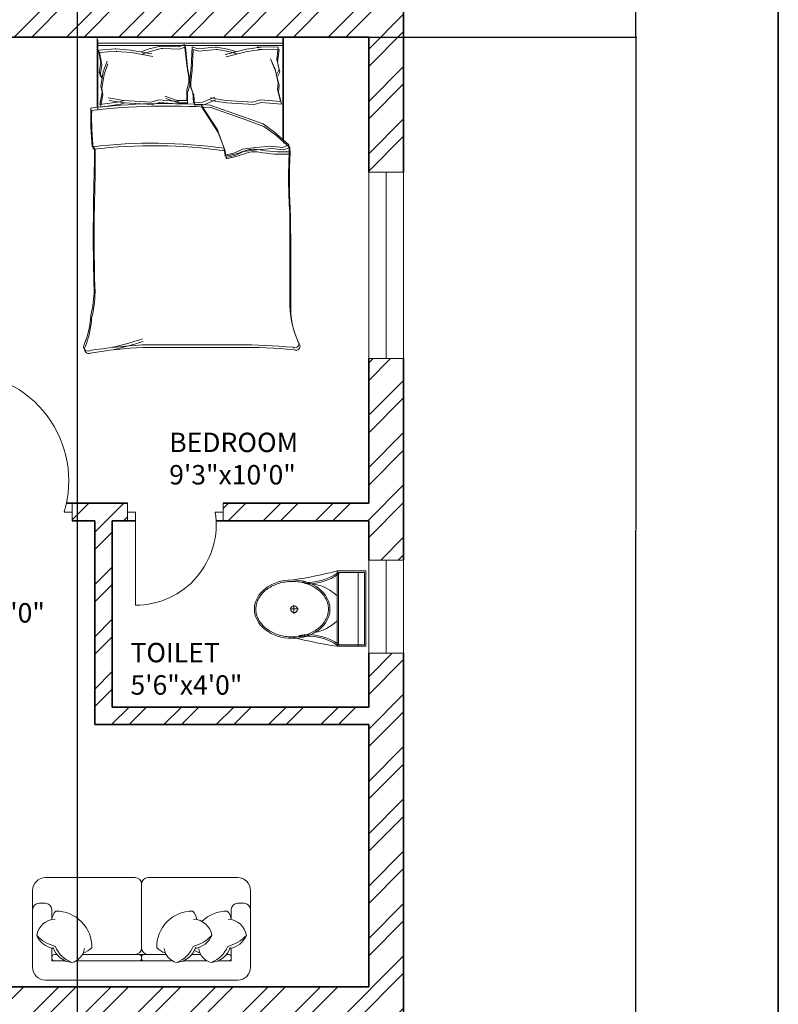
# Model space of a CAD drawing. Units: inches. Extents: x 2552 to 3217, y 1417 to 2737.
# Tile 15 of 25: x 3022 to 3217, y 2138 to 2392. Entities that reach past the tile are written whole.
import ezdxf

# ---------------------------------------------------------------- set-up
doc = ezdxf.new("R2010")
doc.units = ezdxf.units.IN
for name, color, linetype, lineweight in [('A-ANNO-DIMS', 2, 'Continuous', 18), ('A-ANNO-TTLB', 7, 'Continuous', 35), ('A-AREA-IDEN', 7, 'Continuous', 18), ('A-DOOR', 21, 'Continuous', 18), ('A-FLOR-FIXT', 8, 'Continuous', 18), ('A-FURN', 8, 'Continuous', 13), ('A-GLAZ', 161, 'Continuous', 18), ('A-WALL', 7, 'Continuous', 35), ('A-WALL-PATT', 217, 'Continuous', 13)]:
    doc.layers.add(name, color=color, linetype=linetype, lineweight=lineweight)
doc.styles.get("Standard").update_dxf_attribs({"font": 'arial.ttf'})
doc.dimstyles.get("Standard").update_dxf_attribs({"dimtxt": 0.18, "dimasz": 0.18, "dimexe": 0.18, "dimexo": 0.0625, "dimgap": 0.09, "dimtad": 0, "dimtih": 1, "dimtoh": 1, "dimdec": 4, "dimzin": 0, "dimdsep": 46, "dimtxsty": 'Standard', "dimcen": 0.09, "dimadec": 0, "dimazin": 0, "dimtfac": 1, "dimtdec": 4, "dimtofl": 0, "dimtmove": 0, "dimatfit": 3, "dimfxl": 1, "dimtolj": 1, "dimtzin": 0, "dimarcsym": 0})

# ---------------------------------------------------------------- blocks, each defined once
blk = doc.blocks.new('A$C31115884')
for p, q in [((283.1, 497.7), (223.4, 497.7)), ((257.5, 466.4), (257.5, 523.2)), ((0, 200), (0, 0)), ((520, 200), (0, 200)), ((10, 190), (10, 10)), ((510, 190), (10, 190)), ((510, 10), (510, 190)), ((520, 0), (520, 200)), ((510, 54.5), (0, 54.5)), ((10, 10), (510, 10)), ((0, 0), (520, 0))]:
    blk.add_line(p, q)
blk.add_circle((255.6, 496.4), 23.6)
for centre, radius, start, end in [((2777.7, -204.6), 2807, 165.4549, 171.71327), ((3237, 905), 2807, 188.28673, 194.5451), ((-294.5, 403.3), 364.7, 324.20913, 9.34987), ((-294.5, 403.3), 374.7, 324.20913, 9.34987), ((139.5, 406.2), 293.5, 315.84364, 2.65635), ((805.8, 403.3), 374.7, 179.20365, 215.79087), ((805.8, 403.3), 364.7, 170.65013, 215.79087), ((383.6, 406.2), 293.5, 190.27735, 224.15636)]:
    blk.add_arc(centre, radius, start, end)
blk.add_ellipse((256.2, 509.9), major_axis=(0, -260.7), ratio=0.772727)
blk.add_open_spline([(256.2, 259.2), (263.1, 259.2), (270, 259.7), (287.8, 262.3), (298.7, 265.1), (319.9, 273.1), (330.2, 278.4), (350.1, 291.1), (359.7, 298.7), (377.7, 315.9), (386.2, 325.5), (401.7, 346.6), (408.8, 358.1), (421.3, 382.5), (426.8, 395.5), (435.9, 422.4), (439.5, 436.4), (444.8, 465.1), (446.5, 479.7), (447.9, 509.2), (447.6, 524), (445, 553.3), (442.7, 567.8), (436.3, 596), (432.1, 609.7), (421.9, 636), (416, 648.6), (402.5, 672.1), (395, 683), (378.6, 703), (369.8, 712.1), (351.1, 728), (341.3, 734.8), (320.9, 746.2), (310.4, 750.7), (288.9, 757.3), (278, 759.4), (256, 761), (245, 760.6), (223.1, 757.2), (212.3, 754.3), (191.1, 746.1), (180.8, 740.7), (160.9, 727.8), (151.4, 720.1), (133.5, 702.7), (125.1, 693), (109.6, 671.7), (102.6, 660.2), (90.2, 635.7), (84.9, 622.7), (76, 595.6), (72.4, 581.6), (67.2, 552.9), (65.6, 538.2), (64.4, 508.8), (64.8, 494), (67.5, 464.7), (69.9, 450.2), (76.6, 422), (80.8, 408.3), (91.1, 382.2), (97.2, 369.7), (110.8, 346.3), (118.4, 335.4), (134.8, 315.6), (143.7, 306.7), (162.4, 290.9), (172.3, 284.2), (192.8, 273), (203.3, 268.6), (224.8, 262.2), (235.8, 260.2), (249.9, 259.3), (253, 259.2), (256.2, 259.2)], degree=3, knots=[0, 0, 0, 0, 0.110105, 0.110105, 0.285049, 0.285049, 0.459994, 0.459994, 0.634938, 0.634938, 0.809882, 0.809882, 0.984827, 0.984827, 1.159771, 1.159771, 1.334715, 1.334715, 1.50966, 1.50966, 1.684604, 1.684604, 1.859549, 1.859549, 2.034493, 2.034493, 2.209437, 2.209437, 2.384382, 2.384382, 2.559326, 2.559326, 2.73427, 2.73427, 2.909215, 2.909215, 3.084159, 3.084159, 3.259103, 3.259103, 3.434048, 3.434048, 3.608992, 3.608992, 3.783936, 3.783936, 3.958881, 3.958881, 4.133825, 4.133825, 4.30877, 4.30877, 4.483714, 4.483714, 4.658658, 4.658658, 4.833603, 4.833603, 5.008547, 5.008547, 5.183491, 5.183491, 5.358436, 5.358436, 5.53338, 5.53338, 5.708324, 5.708324, 5.883269, 5.883269, 6.058213, 6.058213, 6.233158, 6.233158, 6.283185, 6.283185, 6.283185, 6.283185])
blk = doc.blocks.new('BED-DOUBLE')
for p, q in [((3.47, 63.33), (3.47, 81.44)), ((3.47, 81.44), (51.49, 81.44)), ((3.48, 63.33), (3.48, 81.44)), ((51.27, 81.44), (51.27, 54.83)), ((51.27, 81.44), (51.27, 54.83)), ((51.49, 81.44), (51.49, 80.8)), ((3.47, 79.91), (51.27, 79.91)), ((3.48, 79.91), (51.27, 79.91)), ((3.7, 62.69), (3.7, 80.8)), ((3.7, 62.69), (3.7, 80.8)), ((3.7, 79.27), (51.49, 79.27)), ((3.7, 79.27), (51.49, 79.27)), ((16.88, 78.42), (19.77, 79.14)), ((16.88, 78.42), (19.77, 79.14)), ((19.77, 79.14), (20.09, 79.14)), ((19.77, 79.14), (20.09, 79.14)), ((20.09, 79.14), (24.54, 78.99)), ((20.09, 79.14), (24.54, 78.99)), ((24.54, 78.99), (25.98, 79.57)), ((24.54, 78.99), (25.98, 79.57)), ((24.77, 78.36), (26.21, 78.93)), ((24.77, 78.36), (26.21, 78.93)), ((25.98, 79.57), (26.56, 74.22)), ((25.98, 79.57), (26.56, 74.22)), ((26.21, 78.93), (26.79, 73.58)), ((26.21, 78.93), (26.79, 73.58)), ((27.98, 78.95), (27.73, 73.58)), ((27.98, 78.95), (27.73, 73.58)), ((29.46, 78.46), (27.98, 78.95)), ((29.46, 78.46), (27.98, 78.95)), ((33.88, 78.89), (29.46, 78.46)), ((33.88, 78.89), (29.46, 78.46)), ((34.2, 78.91), (33.88, 78.89)), ((34.2, 78.91), (33.88, 78.89)), ((37.14, 78.36), (34.2, 78.91)), ((37.14, 78.36), (34.2, 78.91)), ((45.71, 78.9), (41.91, 78.37)), ((45.71, 78.9), (41.91, 78.37)), ((50.11, 78.89), (44.71, 78.98)), ((44.71, 78.98), (45.71, 78.9)), ((50.11, 78.89), (44.71, 78.98)), ((44.71, 78.98), (45.71, 78.9)), ((50.11, 78.89), (49.73, 75.68)), ((50.11, 78.89), (49.73, 75.68)), ((51.49, 80.8), (51.49, 54.19)), ((51.49, 80.8), (51.49, 54.19)), ((3.89, 78.13), (4.47, 74.95)), ((3.89, 78.13), (4.47, 74.95)), ((3.9, 78.11), (8.18, 78.43)), ((3.9, 78.11), (8.18, 78.43)), ((4.12, 77.49), (4.7, 74.31)), ((4.12, 77.49), (4.7, 74.31)), ((4.13, 77.47), (8.41, 77.8)), ((4.13, 77.47), (8.41, 77.8)), ((8.18, 78.43), (8.28, 78.42)), ((8.18, 78.43), (8.28, 78.42)), ((8.28, 78.42), (12.11, 78.13)), ((8.28, 78.42), (12.11, 78.13)), ((8.41, 77.8), (8.51, 77.78)), ((8.41, 77.8), (8.51, 77.78)), ((8.51, 77.78), (12.34, 77.49)), ((8.51, 77.78), (12.34, 77.49)), ((12.11, 78.13), (17.6, 77.12)), ((12.11, 78.13), (17.6, 77.12)), ((12.34, 77.49), (17.83, 76.48)), ((12.34, 77.49), (17.83, 76.48)), ((14.85, 77.69), (16.88, 78.42)), ((14.85, 77.69), (16.88, 78.42)), ((15.08, 77.05), (17.11, 77.78)), ((15.08, 77.05), (17.11, 77.78)), ((17.11, 77.78), (20, 78.5)), ((17.11, 77.78), (20, 78.5)), ((20, 78.5), (20.32, 78.5)), ((20, 78.5), (20.32, 78.5)), ((20.32, 78.5), (24.77, 78.36)), ((20.32, 78.5), (24.77, 78.36)), ((28.21, 78.31), (27.96, 72.94)), ((28.21, 78.31), (27.96, 72.94)), ((29.68, 77.83), (28.21, 78.31)), ((29.68, 77.83), (28.21, 78.31)), ((34.11, 78.25), (29.68, 77.83)), ((34.11, 78.25), (29.68, 77.83)), ((34.43, 78.27), (34.11, 78.25)), ((34.43, 78.27), (34.11, 78.25)), ((37.36, 77.73), (34.43, 78.27)), ((37.36, 77.73), (34.43, 78.27)), ((41.91, 78.37), (36.49, 77.02)), ((41.91, 78.37), (36.5, 77.02)), ((42.14, 77.73), (36.72, 76.38)), ((42.14, 77.73), (36.72, 76.38)), ((39.2, 77.77), (37.14, 78.36)), ((39.2, 77.77), (37.14, 78.36)), ((39.43, 77.13), (37.36, 77.73)), ((39.43, 77.13), (37.36, 77.73)), ((45.94, 78.26), (42.14, 77.73)), ((45.94, 78.26), (42.14, 77.73)), ((50.34, 78.25), (44.94, 78.34)), ((44.94, 78.34), (45.94, 78.26)), ((50.34, 78.25), (44.94, 78.34)), ((44.94, 78.34), (45.94, 78.26)), ((50.34, 78.25), (49.96, 75.04)), ((50.34, 78.25), (49.96, 75.04)), ((4.47, 74.95), (4.04, 72.34)), ((4.47, 74.95), (4.04, 72.34)), ((4.7, 74.31), (4.27, 71.7)), ((4.7, 74.31), (4.27, 71.7)), ((5.05, 72.49), (6.06, 75.24)), ((5.05, 72.49), (6.06, 75.24)), ((5.28, 71.85), (6.29, 74.6)), ((5.28, 71.85), (6.29, 74.6)), ((26.56, 74.22), (27.14, 71.04)), ((26.56, 74.22), (27.14, 71.04)), ((26.79, 73.58), (27.37, 70.4)), ((26.79, 73.58), (27.37, 70.4)), ((27.73, 73.58), (27.35, 70.37)), ((27.73, 73.58), (27.35, 70.37)), ((49.31, 73.19), (48.13, 75.86)), ((49.31, 73.19), (48.13, 75.86)), ((49.54, 72.55), (48.36, 75.23)), ((49.54, 72.55), (48.36, 75.23)), ((49.73, 75.68), (50.33, 73.1)), ((49.73, 75.68), (50.33, 73.1)), ((49.96, 75.04), (50.56, 72.47)), ((49.96, 75.04), (50.56, 72.47)), ((4.04, 72.34), (4.62, 71.33)), ((4.04, 72.34), (4.62, 71.33)), ((4.27, 71.7), (4.85, 70.69)), ((4.27, 71.7), (4.85, 70.69)), ((4.47, 68.87), (5.05, 72.49)), ((4.47, 68.87), (5.05, 72.49)), ((4.7, 68.23), (5.28, 71.85)), ((4.7, 68.23), (5.28, 71.85)), ((27.14, 71.04), (27.14, 69.74)), ((27.14, 71.04), (27.14, 69.74)), ((27.96, 72.94), (27.58, 69.73)), ((27.96, 72.94), (27.58, 69.73)), ((50.11, 69.61), (49.31, 73.19)), ((50.11, 69.61), (49.31, 73.19)), ((50.34, 68.98), (49.54, 72.55)), ((50.34, 68.98), (49.54, 72.55)), ((50.33, 73.1), (49.81, 72.06)), ((50.33, 73.1), (49.81, 72.06)), ((50.56, 72.47), (50.04, 71.42)), ((50.56, 72.47), (50.04, 71.42)), ((4.76, 67.28), (4.47, 68.87)), ((4.76, 67.28), (4.47, 68.87)), ((27.14, 69.74), (26.56, 67.86)), ((27.14, 69.74), (26.56, 67.86)), ((27.37, 69.1), (26.79, 67.22)), ((27.37, 69.1), (26.79, 67.22)), ((27.35, 70.37), (27.44, 69.07)), ((27.35, 70.37), (27.44, 69.07)), ((27.37, 70.4), (27.37, 69.1)), ((27.37, 70.4), (27.37, 69.1)), ((27.44, 69.07), (28.13, 67.23)), ((27.44, 69.07), (28.13, 67.23)), ((27.58, 69.73), (27.66, 68.43)), ((27.58, 69.73), (27.66, 68.43)), ((49.92, 68.01), (50.11, 69.61)), ((49.92, 68.01), (50.11, 69.61)), ((50.15, 67.37), (50.34, 68.98)), ((50.15, 67.37), (50.34, 68.98)), ((4.18, 64.1), (4.76, 67.28)), ((4.18, 64.1), (4.76, 67.28)), ((4.41, 63.46), (4.99, 66.64)), ((4.41, 63.46), (4.99, 66.64)), ((4.99, 66.64), (4.7, 68.23)), ((4.99, 66.64), (4.7, 68.23)), ((24.1, 65.18), (20.96, 66.27)), ((24.1, 65.18), (20.96, 66.27)), ((26.56, 67.86), (26.56, 65.18)), ((26.56, 67.86), (26.56, 65.18)), ((26.79, 67.22), (26.79, 64.54)), ((26.79, 67.22), (26.79, 64.54)), ((27.66, 68.43), (28.36, 66.59)), ((27.66, 68.43), (28.36, 66.59)), ((28.13, 67.23), (28.3, 64.55)), ((28.13, 67.23), (28.3, 64.55)), ((28.36, 66.59), (28.53, 63.91)), ((28.36, 66.59), (28.53, 63.91)), ((30.75, 64.7), (33.82, 65.99)), ((30.75, 64.7), (33.82, 65.99)), ((50.7, 64.87), (49.92, 68.01)), ((50.7, 64.87), (49.92, 68.01)), ((50.93, 64.23), (50.15, 67.37)), ((50.93, 64.23), (50.15, 67.37)), ((9.28, 64.83), (4.18, 64.1)), ((9.28, 64.83), (4.18, 64.1)), ((9.51, 64.19), (4.41, 63.46)), ((9.51, 64.19), (4.41, 63.46)), ((6.38, 65.81), (10.41, 65.15)), ((6.38, 65.81), (10.41, 65.15)), ((6.61, 65.18), (10.64, 64.51)), ((6.61, 65.18), (10.64, 64.51)), ((10.41, 65.15), (9.28, 64.83)), ((10.41, 65.15), (9.28, 64.83)), ((10.64, 64.51), (9.51, 64.19)), ((10.64, 64.51), (9.51, 64.19)), ((10.41, 65.15), (17.42, 64.72)), ((10.41, 65.15), (17.42, 64.72)), ((10.64, 64.51), (17.65, 64.08)), ((10.64, 64.51), (17.65, 64.08)), ((17.42, 64.72), (19.38, 65.27)), ((17.42, 64.72), (19.38, 65.27)), ((17.65, 64.08), (19.61, 64.63)), ((17.65, 64.08), (19.61, 64.63)), ((19.38, 65.27), (24.52, 64.87)), ((19.38, 65.27), (24.52, 64.87)), ((19.61, 64.63), (24.74, 64.23)), ((19.61, 64.63), (24.74, 64.23)), ((24.33, 64.54), (21.19, 65.63)), ((24.33, 64.54), (21.19, 65.63)), ((26.56, 65.18), (24.1, 65.18)), ((26.56, 65.18), (24.1, 65.18)), ((26.79, 64.54), (24.33, 64.54)), ((26.79, 64.54), (24.33, 64.54)), ((28.3, 64.55), (30.75, 64.7)), ((28.3, 64.55), (30.75, 64.7)), ((28.53, 63.91), (30.98, 64.06)), ((28.53, 63.91), (30.98, 64.06)), ((30.26, 64.06), (34.45, 57.57)), ((30.26, 64.06), (34.45, 57.57)), ((30.49, 63.42), (34.68, 56.93)), ((30.49, 63.42), (34.68, 56.93)), ((30.98, 64.06), (34.05, 65.35)), ((30.98, 64.06), (34.05, 65.35)), ((40.64, 61.13), (32.31, 64.06)), ((40.64, 61.13), (32.31, 64.06)), ((40.87, 60.49), (32.53, 63.42)), ((40.87, 60.49), (32.53, 63.42)), ((32.56, 65.81), (36.6, 65.15)), ((32.56, 65.81), (36.6, 65.15)), ((32.79, 65.18), (36.82, 64.51)), ((32.79, 65.18), (36.82, 64.51)), ((36.6, 65.15), (43.61, 64.72)), ((36.6, 65.15), (43.61, 64.72)), ((36.82, 64.51), (43.83, 64.08)), ((36.82, 64.51), (43.83, 64.08)), ((43.61, 64.72), (45.57, 65.27)), ((43.61, 64.72), (45.57, 65.27)), ((43.83, 64.08), (45.79, 64.63)), ((43.83, 64.08), (45.79, 64.63)), ((45.57, 65.27), (50.7, 64.87)), ((45.57, 65.27), (50.7, 64.87)), ((45.79, 64.63), (50.93, 64.23)), ((45.79, 64.63), (50.93, 64.23)), ((46.22, 59.11), (40.64, 61.13)), ((46.22, 59.11), (40.64, 61.13)), ((46.45, 58.48), (40.87, 60.49)), ((46.45, 58.48), (40.87, 60.49)), ((49.16, 56.95), (46.22, 59.11)), ((49.16, 56.95), (46.22, 59.11)), ((49.39, 56.31), (46.45, 58.48)), ((49.39, 56.31), (46.45, 58.48)), ((34.45, 57.57), (36.15, 53.08)), ((34.45, 57.57), (36.15, 53.08)), ((34.68, 56.93), (36.38, 52.44)), ((34.68, 56.93), (36.38, 52.44)), ((52.87, 53.7), (49.16, 56.95)), ((52.87, 53.7), (49.16, 56.95)), ((53.1, 53.06), (49.39, 56.31)), ((53.1, 53.06), (49.39, 56.31)), ((44.36, 53.08), (48.23, 53.39)), ((44.36, 53.08), (48.23, 53.39)), ((48.23, 53.39), (51.33, 53.08)), ((48.23, 53.39), (51.33, 53.08)), ((51.33, 53.08), (52.87, 53.7)), ((51.33, 53.08), (52.87, 53.7)), ((52.95, 51.95), (52.87, 53.7, 3.87)), ((52.95, 51.95), (52.87, 53.7, 3.87)), ((36.15, 53.08), (36.46, 51.07)), ((36.15, 53.08), (36.46, 51.07)), ((36.38, 52.44), (36.69, 50.43)), ((36.38, 52.44), (36.69, 50.43)), ((36.46, 51.07), (38.94, 51.69)), ((36.46, 51.07), (38.94, 51.69)), ((36.69, 50.43), (39.17, 51.05)), ((36.69, 50.43), (39.17, 51.05)), ((38.94, 51.69), (40.95, 52.61)), ((38.94, 51.69), (40.95, 52.61)), ((39.17, 51.05), (41.18, 51.97)), ((39.17, 51.05), (41.18, 51.97)), ((40.95, 52.61), (44.36, 53.08)), ((40.95, 52.61), (44.36, 53.08)), ((41.18, 51.97), (44.59, 52.44)), ((41.18, 51.97), (44.59, 52.44)), ((44.59, 52.44), (48.46, 52.75)), ((44.59, 52.44), (48.46, 52.75)), ((48.46, 52.75), (51.56, 52.44)), ((48.46, 52.75), (51.56, 52.44)), ((51.56, 52.44), (53.1, 53.06)), ((51.56, 52.44), (53.1, 53.06)), ((53.18, 51.31), (53.1, 53.06, 3.87)), ((53.18, 51.31), (53.1, 53.06, 3.87)), ((15.06, 2.2), (39.68, 2.2)), ((15.06, 2.2), (39.68, 2.2)), ((15.29, 1.56), (39.91, 1.56)), ((15.29, 1.56), (39.91, 1.56))]:
    blk.add_line(p, q)
for centre, radius, start, end in [((21.36, -100.61), 164.97, 86.0865, 96.7821), ((21.36, -100.61), 164.97, 86.0865, 96.7821), ((21.59, -101.25), 164.97, 86.0865, 96.7821), ((21.59, -101.25), 164.97, 86.0865, 96.7821), ((85.16, 61.35), 83.31, 178.7218, 185.604), ((85.16, 61.35), 83.31, 178.7218, 185.604), ((85.39, 60.71), 83.31, 178.7218, 185.604), ((85.39, 60.71), 83.31, 178.7218, 185.604), ((17.76, -74.87), 129.02, 81.7845, 96.9006), ((17.76, -74.87), 129.02, 81.7845, 96.9006), ((17.98, -75.51), 129.02, 81.7845, 96.9006), ((17.98, -75.51), 129.02, 81.7845, 96.9006), ((-167.31, 50.27), 170.11, 358.4762, 1.0082), ((-167.31, 50.27), 170.11, 358.4762, 1.0082), ((-167.08, 49.63), 170.11, 358.4762, 1.0082), ((-167.08, 49.63), 170.11, 358.4762, 1.0082), ((36.64, 51), 0.185, 160.2464, 271.1377), ((36.64, 51), 0.185, 160.2464, 271.1377), ((31.15, 79.96), 29.65, 280.6617, 289.8806), ((31.15, 79.96), 29.65, 280.6617, 289.8806), ((31.38, 79.32), 29.65, 280.6617, 289.8806), ((31.38, 79.32), 29.65, 280.6617, 289.8806), ((43.74, 46.38), 6.22, 78.6608, 113.7384), ((43.74, 46.38), 6.22, 78.6608, 113.7384), ((43.97, 45.74), 6.22, 78.6608, 113.7384), ((43.97, 45.74), 6.22, 78.6608, 113.7384), ((51.33, 88.1), 36.18, 259.8763, 272.5657), ((51.33, 88.1), 36.18, 259.8763, 272.5657), ((51.56, 87.46), 36.18, 259.8763, 272.5657), ((51.56, 87.46), 36.18, 259.8763, 272.5657), ((182.27, 45.13), 129.5, 176.9791, 183.8365), ((182.27, 45.13), 129.5, 176.9791, 183.8365), ((182.49, 44.49), 129.5, 176.9791, 183.8365), ((182.49, 44.49), 129.5, 176.9791, 183.8365), ((36.86, 50.36), 0.185, 160.2464, 271.1377), ((36.86, 50.36), 0.185, 160.2464, 271.1377), ((484.82, 30.83), 482.31, 178.2277, 181.7185), ((484.82, 30.83), 482.31, 178.2277, 181.7185), ((485.05, 30.19), 482.31, 178.2277, 181.7185), ((485.05, 30.19), 482.31, 178.2277, 181.7185), ((-4508.74, 13.62), 4561.86, 0.00217, 0.28689), ((-4508.74, 13.62), 4561.86, 0.00217, 0.28689), ((-4508.51, 12.98), 4561.86, 0.00217, 0.28689), ((-4508.52, 12.98), 4561.86, 0.00217, 0.28689), ((-26.9, 16.93), 29.63, 346.0648, 358.9113), ((-26.9, 16.93), 29.63, 346.0648, 358.9113), ((-26.67, 16.29), 29.63, 346.0648, 358.9113), ((-26.67, 16.29), 29.63, 346.0648, 358.9113), ((76.16, 12.78), 23.07, 177.4714, 206.4681), ((76.16, 12.78), 23.07, 177.4714, 206.4681), ((76.39, 12.14), 23.07, 177.4714, 206.4681), ((76.39, 12.14), 23.07, 177.4714, 206.4681), ((-21.66, 11.17), 23.56, 337.9751, 356.652), ((-21.66, 11.17), 23.56, 337.9751, 356.652), ((-21.43, 10.53), 23.56, 337.9751, 356.652), ((-21.43, 10.53), 23.56, 337.9751, 356.652), ((-17.22, 105.16), 106.46, 283.3832, 287.7053), ((-17.22, 105.16), 106.46, 283.3832, 287.7053), ((-16.99, 104.52), 106.46, 283.3832, 287.7053), ((-16.99, 104.52), 106.46, 283.3832, 287.7053), ((1.09, 1.73), 1.09, 146.1736, 293.4781), ((1.09, 1.73), 1.09, 146.1736, 293.4781), ((1.32, 1.09), 1.09, 146.1736, 293.4781), ((1.32, 1.09), 1.09, 146.1736, 293.4781), ((21.43, -119.39), 121.76, 92.9958, 99.4091), ((21.43, -119.39), 121.76, 92.9958, 99.4091), ((21.66, -120.03), 121.76, 92.9958, 99.4091), ((21.65, -120.03), 121.76, 92.9958, 99.4091), ((41.15, -130.83), 133.04, 84.4998, 90.6351), ((41.15, -130.83), 133.04, 84.4998, 90.6351), ((41.38, -131.47), 133.04, 84.4998, 90.6351), ((41.38, -131.47), 133.04, 84.4998, 90.6351), ((54.41, 2.57), 1.1, 242.6588, 356.02), ((54.41, 2.57), 1.1, 242.6588, 356.02), ((54.64, 1.93), 1.1, 242.6588, 356.02), ((54.64, 1.93), 1.1, 242.6588, 356.02)]:
    blk.add_arc(centre, radius, start, end)
blk = doc.blocks.new('WIN-48')
for p, q in [((4.5, 48), (0, 48)), ((0, 48), (9, 48)), ((0, 48), (0, 0)), ((4.5, 0), (4.5, 48)), ((9, 48), (9, 0)), ((0, 0), (9, 0)), ((9, 0), (4.5, 0))]:
    blk.add_line(p, q)
blk = doc.blocks.new('WIN-24')
for p, q in [((0, 24), (9, 24)), ((0, 24), (0, 0)), ((9, 24), (4.5, 24)), ((4.5, 24), (4.5, 0)), ((9, 24), (9, 0)), ((4.5, 0), (0, 0)), ((0, 0), (9, 0))]:
    blk.add_line(p, q)
blk = doc.blocks.new('*D54')
at = {"layer": 'A-ANNO-DIMS', "color": 0, "lineweight": -2, "transparency": 16777216}
for p, q in [((3111.42, 2387.01), (3180.33, 2387.01)), ((3180.15, 2386.83), (3180.15, 2260.44)), ((3180.15, 2133.69), (3180.15, 2260.08)), ((3111.42, 2133.51), (3180.33, 2133.51))]:
    blk.add_line(p, q, dxfattribs=at)
at = {"layer": 'A-ANNO-DIMS', "color": 0, "transparency": 16777216}
for points in [[(3180.12, 2386.83), (3180.18, 2386.83), (3180.15, 2387.01)], [(3180.12, 2133.69), (3180.18, 2133.69), (3180.15, 2133.51)]]:
    blk.add_solid(points, dxfattribs=at)
at = {"layer": 'Defpoints', "color": 0, "transparency": 16777216}
for p in [(3111.35, 2387.01), (3180.15, 2387.01), (3111.35, 2133.51)]:
    blk.add_point(p, dxfattribs=at)
at = {"layer": 'A-ANNO-DIMS', "color": 0, "transparency": 16777216, "insert": (3180.15, 2260.26), "char_height": 0.18, "attachment_point": 5}
blk.add_mtext('\\A1;253.5', dxfattribs=at)
blk = doc.blocks.new('*D57')
at = {"layer": 'A-ANNO-DIMS', "color": 0, "lineweight": -2, "transparency": 16777216}
for p, q in [((3004.08, 2515.95), (3004.08, 1482.53)), ((3036.34, 2515.95), (3036.34, 1482.53)), ((3004.26, 1482.71), (3019.75, 1482.71)), ((3036.16, 1482.71), (3020.68, 1482.71))]:
    blk.add_line(p, q, dxfattribs=at)
at = {"layer": 'A-ANNO-DIMS', "color": 0, "transparency": 16777216}
for points in [[(3004.26, 1482.74), (3004.26, 1482.68), (3004.08, 1482.71)], [(3036.16, 1482.74), (3036.16, 1482.68), (3036.34, 1482.71)]]:
    blk.add_solid(points, dxfattribs=at)
at = {"layer": 'Defpoints', "color": 0, "transparency": 16777216}
for p in [(3004.08, 2516.01), (3036.34, 2516.01), (3036.34, 1482.71)]:
    blk.add_point(p, dxfattribs=at)
at = {"layer": 'A-ANNO-DIMS', "color": 0, "transparency": 16777216, "insert": (3020.21, 1482.71), "char_height": 0.18, "attachment_point": 5}
blk.add_mtext('\\A1;32.255', dxfattribs=at)
blk = doc.blocks.new('*D66')
at = {"layer": 'A-ANNO-DIMS', "color": 0, "lineweight": -2, "transparency": 16777216}
for p, q in [((3120.42, 2481.18), (3180.33, 2481.18)), ((3180.15, 2481), (3180.15, 2434.28)), ((3180.15, 2387.19), (3180.15, 2433.92)), ((3111.42, 2387.01), (3180.33, 2387.01))]:
    blk.add_line(p, q, dxfattribs=at)
at = {"layer": 'A-ANNO-DIMS', "color": 0, "transparency": 16777216}
for points in [[(3180.12, 2481), (3180.18, 2481), (3180.15, 2481.18)], [(3180.12, 2387.19), (3180.18, 2387.19), (3180.15, 2387.01)]]:
    blk.add_solid(points, dxfattribs=at)
at = {"layer": 'Defpoints', "color": 0, "transparency": 16777216}
for p in [(3120.35, 2481.18), (3111.35, 2387.01), (3180.15, 2387.01)]:
    blk.add_point(p, dxfattribs=at)
at = {"layer": 'A-ANNO-DIMS', "color": 0, "transparency": 16777216, "insert": (3180.15, 2434.1), "char_height": 0.18, "attachment_point": 5}
blk.add_mtext('\\A1;94.17', dxfattribs=at)

msp = doc.modelspace()

# ---------------------------------------------------------------- hatches: boundary and pattern name
at = {"layer": 'A-WALL-PATT'}
h = msp.add_hatch(dxfattribs=at)
h.set_pattern_fill('ANSI32', color=256)
h.paths.add_polyline_path([(2756.676, 2649.5125), (2637.3535, 2649.5125), (2637.3535, 2617.9626), (2641.8535, 2617.9626), (2646.3535, 2617.9626), (2646.3535, 2640.5125), (2724.3535, 2640.5125), (2724.3535, 2520.5125), (2720.299, 2520.5125), (2720.299, 2516.0125), (2733.4075, 2516.0125), (2733.4075, 2518.2213), (2733.4075, 2520.5125), (2728.8535, 2520.5125), (2728.8535, 2640.5125), (2756.676, 2640.5125)])
h.paths.add_polyline_path([(2848.8535, 2649.5125), (2804.676, 2649.5125), (2804.676, 2640.5125), (2839.8535, 2640.5125), (2839.8535, 2598.3517), (2848.8535, 2598.3517)])
h.paths.add_polyline_path([(2646.3535, 2516.0125), (2697.9593, 2516.0125), (2697.9593, 2518.2625), (2697.9593, 2520.5125), (2646.3535, 2520.5125), (2646.3535, 2581.9626), (2637.3535, 2581.9626), (2637.3535, 2364.3298), (2646.3535, 2364.3298), (2646.3535, 2387.0125), (2724.3535, 2387.0125), (2724.3535, 2267.0125), (2721.0443, 2267.0125), (2721.0443, 2262.5125), (2733.7854, 2262.5125), (2733.7854, 2264.7625), (2733.7854, 2267.0125), (2728.8535, 2267.0125), (2728.8535, 2387.0125), (2839.8535, 2387.0125), (2839.8535, 2363.8387), (2848.8535, 2363.8387), (2848.8535, 2403.7415), (2844.3535, 2403.7415), (2839.8535, 2403.7415), (2839.8535, 2396.0125), (2646.3535, 2396.0125)])
h.paths.add_polyline_path([(2848.8535, 2550.3517), (2844.3535, 2550.3517), (2839.8535, 2550.3517), (2839.8535, 2520.5125), (2801.9195, 2520.5125), (2801.9195, 2518.2625), (2801.9195, 2516.0125), (2839.8535, 2516.0125), (2839.8535, 2507.5813), (2848.8535, 2507.5813)], flags=17)
h.paths.add_polyline_path([(2848.8535, 2483.5813), (2844.3535, 2483.5813), (2839.8535, 2483.5813), (2839.8535, 2468.0125), (2773.8535, 2468.0125), (2773.8535, 2516.0125), (2778.1336, 2516.0125), (2778.1336, 2520.5125), (2766.696, 2520.5125), (2766.696, 2518.2625), (2766.696, 2516.0125), (2769.3535, 2516.0125), (2769.3535, 2463.5125), (2839.8535, 2463.5125), (2839.8535, 2431.0782), (2848.8535, 2431.0782)], flags=17)
h.paths.add_polyline_path([(2917.8535, 2569.2764), (2913.3535, 2569.2764), (2908.8535, 2569.2764), (2908.8535, 2433.001), (2917.8535, 2433.001), (2917.8535, 2516.0125), (2967.486, 2516.0125), (2967.486, 2520.5125), (2917.8535, 2520.5125)])
h.paths.add_polyline_path([(3000.3535, 2640.5125), (2995.8535, 2640.5125), (2995.8535, 2520.5125), (2990.688, 2520.5125), (2990.688, 2516.0125), (3004.0844, 2516.0125), (3004.0844, 2518.2625), (3004.0844, 2520.5125), (3000.3535, 2520.5125)])
h.paths.add_polyline_path([(3120.3535, 2561.3689), (3115.8535, 2561.3689), (3111.3535, 2561.3689), (3111.3535, 2520.5125), (3070.9814, 2520.5125), (3070.9814, 2518.2625), (3070.9814, 2516.0125), (3111.3535, 2516.0125), (3111.3535, 2505.1841), (3120.3535, 2505.1841)])
h.paths.add_polyline_path([(3120.3535, 2481.1841), (3115.8535, 2481.1841), (3111.3535, 2481.1841), (3111.3535, 2468.0125), (3045.3535, 2468.0125), (3045.3535, 2516.0125), (3048.9787, 2516.0125), (3048.9787, 2520.5125), (3036.3395, 2520.5125), (3036.3395, 2516.0125), (3040.8535, 2516.0125), (3040.8535, 2463.5125), (3111.3535, 2463.5125), (3111.3535, 2396.0125), (2917.8535, 2396.0125), (2917.8535, 2403.4124), (2913.3535, 2403.4124), (2908.8535, 2403.4124), (2908.8535, 2182.5756), (2917.8535, 2182.5756), (2917.8535, 2262.5125), (2968.001, 2262.5125), (2968.001, 2264.7625), (2968.001, 2267.0125), (2917.8535, 2267.0125), (2917.8535, 2387.0125), (3111.3535, 2387.0125), (3111.3535, 2352.2435), (3120.3535, 2352.2435)])
h.paths.add_polyline_path([(3120.3535, 2304.2435), (3115.8535, 2304.2435), (3111.3535, 2304.2435), (3111.3535, 2267.0125), (3073.8616, 2267.0125), (3073.8616, 2264.7625), (3073.8616, 2262.5125), (3111.3535, 2262.5125), (3111.3535, 2252.376), (3120.3535, 2252.376)], flags=17)
h.paths.add_polyline_path([(3120.3535, 2228.376), (3115.8535, 2228.376), (3111.3535, 2228.376), (3111.3535, 2214.5125), (3045.3535, 2214.5125), (3045.3535, 2262.5125), (3049.3096, 2262.5125), (3049.3096, 2267.0125), (3035.0125, 2267.0125), (3035.0125, 2262.5125), (3040.8535, 2262.5125), (3040.8535, 2210.0125), (3111.3535, 2210.0125), (3111.3535, 2142.5125), (2917.8535, 2142.5125), (2917.8535, 2150.2408), (2913.3535, 2150.2408), (2908.8535, 2150.2408), (2908.8535, 1924.9905), (2917.8535, 1924.9905), (2917.8535, 2009.0125), (2971.959, 2009.0125), (2971.959, 2011.2625), (2971.959, 2013.5125), (2917.8535, 2013.5125), (2917.8535, 2133.5125), (2995.8535, 2133.5125), (2995.8535, 2013.5125), (2992.1797, 2013.5125), (2992.1797, 2009.0125), (3004.3344, 2009.0125), (3004.3344, 2011.2625), (3004.3344, 2013.5125), (3000.3535, 2013.5125), (3000.3535, 2133.5125), (3111.3535, 2133.5125), (3111.3535, 2115.0291), (3120.3535, 2115.0291)])
h.paths.add_polyline_path([(3000.3535, 2387.0125), (2995.8535, 2387.0125), (2995.8535, 2267.0125), (2991.3326, 2267.0125), (2991.3326, 2262.5125), (3004.1044, 2262.5125), (3004.1044, 2264.7625), (3004.1044, 2267.0125), (3000.3535, 2267.0125)], flags=17)
h.paths.add_polyline_path([(3120.3535, 1973.2388), (3115.8535, 1973.2388), (3111.3535, 1973.2388), (3111.3535, 1961.0125), (3045.3535, 1961.0125), (3045.3535, 2009.0125), (3048.9101, 2009.0125), (3048.9101, 2013.5125), (3037.105, 2013.5125), (3037.105, 2011.2625), (3037.105, 2009.0125), (3040.8535, 2009.0125), (3040.8535, 1956.5125), (3111.3535, 1956.5125), (3111.3535, 1889.0125), (2917.8535, 1889.0125), (2917.8535, 1895.7215), (2913.3535, 1895.7215), (2908.8535, 1895.7215), (2908.8535, 1844.2217), (2917.8535, 1844.2217), (2917.8535, 1880.0125), (3111.3535, 1880.0125), (3111.3535, 1846.9541), (3120.3535, 1846.9541)])
h.paths.add_polyline_path([(3120.3535, 2067.0291), (3111.3535, 2067.0291), (3111.3535, 2013.5125), (3071.3001, 2013.5125), (3071.3001, 2009.0125), (3111.3535, 2009.0125), (3111.3535, 1997.2388), (3120.3535, 1997.2388)], flags=0)
h.paths.add_polyline_path([(3120.3535, 1798.9541), (3115.8535, 1798.9541), (3111.3535, 1798.9541), (3111.3535, 1760.0125), (3071.2497, 1760.0125), (3071.2497, 1757.7625), (3071.2497, 1755.5125), (3111.3535, 1755.5125), (3111.3535, 1746.162), (3120.3535, 1746.2478)])
h.paths.add_polyline_path([(3120.3535, 1722.2049), (3111.3535, 1722.2049), (3111.3535, 1707.5125), (3045.3535, 1707.5125), (3045.3535, 1755.5125), (3048.6624, 1755.5125), (3048.6624, 1760.0125), (3035.3703, 1760.0125), (3035.3703, 1755.5125), (3040.8535, 1755.5125), (3040.8535, 1703.0125), (3111.3535, 1703.0125), (3111.3535, 1635.5125), (2917.8535, 1635.5125), (2917.8535, 1643.1366), (2913.3535, 1643.1366), (2908.8535, 1643.1366), (2908.8535, 1626.5125), (3120.3535, 1626.5125)])
h.paths.add_polyline_path([(2917.8535, 1755.5125), (2973.2287, 1755.5125), (2973.2287, 1757.7625), (2973.2287, 1760.0125), (2917.8535, 1760.0125), (2917.8535, 1808.2217), (2913.3535, 1808.2217), (2908.8535, 1808.2217), (2908.8535, 1676.1665), (2917.8535, 1676.1665)])
h.paths.add_polyline_path([(3000.3535, 1880.0125), (2995.8535, 1880.0125), (2995.8535, 1760.0125), (2992.9329, 1760.0125), (2992.9329, 1755.5125), (3003.8766, 1755.5125), (3003.8766, 1757.7625), (3003.8766, 1760.0125), (3000.3535, 1760.0125)])
h.paths.add_polyline_path([(2848.8535, 1896.6971), (2844.3535, 1896.6971), (2839.8535, 1896.6971), (2839.8535, 1889.0125), (2646.3535, 1889.0125), (2646.3535, 2009.0125), (2700.5253, 2009.0125), (2700.5253, 2011.2625), (2700.5253, 2013.5125), (2646.3535, 2013.5125), (2646.3535, 2053.1812), (2641.8535, 2053.1812), (2637.3535, 2053.1812), (2637.3535, 1836.254), (2646.3535, 1836.254), (2646.3535, 1880.0125), (2724.3535, 1880.0125), (2724.3535, 1760.0125), (2721.2473, 1760.0125), (2721.2473, 1755.5125), (2731.9187, 1755.5125), (2731.9187, 1757.7625), (2731.9187, 1760.0125), (2728.8535, 1760.0125), (2728.8535, 1880.0125), (2839.8535, 1880.0125), (2839.8535, 1840.3813), (2848.8535, 1840.3813)])
h.paths.add_polyline_path([(2848.8535, 1792.3813), (2844.3535, 1792.3813), (2839.8535, 1792.3813), (2839.8535, 1760.0125), (2797.8845, 1760.0125), (2797.8845, 1755.5125), (2839.8535, 1755.5125), (2839.8535, 1743.3688), (2844.3535, 1743.3688), (2848.8535, 1743.3688)], flags=0)
h.paths.add_polyline_path([(2848.8535, 1719.3688), (2844.3535, 1719.3688), (2839.8535, 1719.3688), (2839.8535, 1707.5125), (2773.8535, 1707.5125), (2773.8535, 1755.5125), (2777.716, 1755.5125), (2777.716, 1760.0125), (2760.9247, 1760.0125), (2760.9247, 1757.9721), (2760.9247, 1755.5125), (2769.3535, 1755.5125), (2769.3535, 1703.0125), (2839.8535, 1703.0125), (2839.8535, 1673.0277), (2848.8535, 1672.9407)], flags=0)
h.paths.add_polyline_path([(2646.3535, 1755.5125), (2702.9171, 1755.5125), (2702.9171, 1757.7625), (2702.9171, 1760.0125), (2646.3535, 1760.0125), (2646.3535, 1800.254), (2641.8535, 1800.254), (2637.3535, 1800.254), (2637.3535, 1626.5125), (2848.8535, 1626.5125), (2848.8535, 1643.1187), (2844.3535, 1643.1187), (2839.8535, 1643.1187), (2839.8535, 1635.5125), (2646.3535, 1635.5125)])
h.paths.add_polyline_path([(2848.8535, 2148.8427), (2844.3535, 2148.8427), (2839.8535, 2148.8427), (2839.8535, 2142.5125), (2646.3535, 2142.5125), (2646.3535, 2262.5125), (2701.3562, 2262.5125), (2701.3562, 2264.7625), (2701.3562, 2267.0125), (2646.3535, 2267.0125), (2646.3535, 2328.3298), (2637.3535, 2328.3298), (2637.3535, 2089.1812), (2646.3535, 2089.1812), (2646.3535, 2133.5125), (2839.8535, 2133.5125), (2839.8535, 2097.5966), (2848.8535, 2097.5966)])
h.paths.add_polyline_path([(2728.8535, 2133.5125), (2724.3535, 2133.5125), (2724.3535, 2013.5125), (2719.6039, 2013.5125), (2719.6039, 2009.0125), (2732.5784, 2009.0125), (2732.5784, 2011.2625), (2732.5784, 2013.5125), (2728.8535, 2013.5125)])
h.paths.add_polyline_path([(2848.8535, 1970.0557), (2844.3535, 1970.0557), (2839.8535, 1970.0557), (2839.8535, 1961.0125), (2773.8535, 1961.0125), (2773.8535, 2009.0125), (2777.3388, 2009.0125), (2777.3388, 2013.5125), (2764.7681, 2013.5125), (2764.7681, 2009.0125), (2769.3535, 2009.0125), (2769.3535, 1956.5125), (2839.8535, 1956.5125), (2839.8535, 1924.7199), (2848.8535, 1924.7199)], flags=17)
h.paths.add_polyline_path([(2848.8535, 2049.5966), (2844.3535, 2049.5966), (2839.8535, 2049.5966), (2839.8535, 2013.5125), (2798.198, 2013.5125), (2798.198, 2011.2625), (2798.198, 2009.0125), (2839.8535, 2009.0125), (2839.8535, 1994.0557), (2848.8535, 1994.0557)], flags=17)
h.paths.add_polyline_path([(2848.8535, 2315.8387), (2839.8535, 2315.8387), (2839.8535, 2267.0125), (2799.3375, 2267.0125), (2799.3375, 2264.7625), (2799.3375, 2262.5125), (2839.8535, 2262.5125), (2839.8535, 2253.2843), (2848.8535, 2253.2843)], flags=17)
h.paths.add_polyline_path([(2848.8535, 2229.2843), (2839.8535, 2229.2843), (2839.8535, 2177.6936), (2848.8535, 2177.6936)], flags=17)
h.paths.add_polyline_path([(2839.8535, 2214.5125), (2773.8535, 2214.5125), (2773.8535, 2262.5125), (2777.6984, 2262.5125), (2777.6984, 2267.0125), (2763.8226, 2267.0125), (2763.8226, 2262.5125), (2769.3535, 2262.5125), (2769.3535, 2210.0125), (2839.8535, 2210.0125)], flags=17)
h.paths.add_polyline_path([(3050.32, 2520.2817), (3088.9114, 2520.2817), (3088.9114, 2538.939), (3050.32, 2538.939)], flags=9)

# ---------------------------------------------------------------- linework, layer by layer
at = {"layer": 'A-ANNO-TTLB'}
msp.add_lwpolyline([(2552.473, 2736.5692), (3216.7862, 2736.5692), (3216.7862, 1416.6914), (2552.473, 1416.6914)], close=True, dxfattribs=at)
at = {"layer": 'A-DOOR'}
for p, q in [((3035.0125, 2267.0125), (3035.0125, 2262.5125)), ((3049.3096, 2262.5125), (3049.3096, 2267.0125)), ((3049.3096, 2267.0125), (3049.3096, 2264.7625)), ((3073.8616, 2262.5125), (3073.8616, 2267.0125)), ((3073.8616, 2267.0125), (3073.8616, 2264.7625)), ((3035.0125, 2264.7625), (3033.0125, 2264.7625)), ((3035.0125, 2262.5125), (3035.0125, 2264.7625)), ((3049.3096, 2264.7625), (3051.3096, 2264.7625)), ((3051.3096, 2264.7625), (3051.3096, 2240.7625)), ((3073.8616, 2264.7625), (3071.8616, 2264.7625))]:
    msp.add_line(p, q, dxfattribs=at)
for centre, radius, start, end in [((3006.1044, 2272.7064), 28.0562, 343.552291, 90), ((3051.3096, 2261.5622), 20.7997, 270, 8.850889)]:
    msp.add_arc(centre, radius, start, end, dxfattribs=at)
at = {"layer": 'A-FURN', "ltscale": 0.03}
msp.add_lwpolyline([(3051.239, 2170.6308, -0.41421356), (3052.8885, 2168.9812, -0.41421356), (3054.5381, 2170.6308), (3077.632, 2170.6308, -0.41421356), (3080.9311, 2167.3316), (3080.9311, 2147.5369, -0.41421356), (3077.632, 2144.2378), (3028.1451, 2144.2378, -0.41421356), (3024.8459, 2147.5369), (3024.8459, 2167.3316, -0.41421356), (3028.1451, 2170.6308), (3051.239, 2170.6308, -0.41421356), (3052.8885, 2168.9812, -0.41421356), (3054.5381, 2170.6308)], format="xyb", dxfattribs=at)
at = {"layer": 'A-FURN'}
for points in [[(3051.239, 2150.836, 0.41421356), (3052.8885, 2152.4856), (3052.8885, 2168.9812, 0.41421356)], [(3054.5381, 2150.836, -0.41421356), (3052.8885, 2152.4856), (3052.8885, 2168.9812, -0.41421356)], [(3024.8459, 2162.3829, -0.41421356), (3026.4955, 2164.0325), (3028.1451, 2164.0325, -0.41421356), (3029.7946, 2162.3829), (3029.7946, 2159.8272)], [(3075.9824, 2159.8272), (3075.9824, 2162.3829, -0.41421356), (3077.632, 2164.0325), (3079.2815, 2164.0325, -0.41421356), (3080.9311, 2162.3829)], [(3030.6224, 2159.927, 0.35677236), (3025.8958, 2155.7691, 0.24954205), (3030.1786, 2152.3426, -9.61688035)], [(3029.791, 2159.8264, -0.16554063), (3030.8115, 2162.006, -0.42598917), (3040.0758, 2152.5562, -0.12152332), (3037.8766, 2151.2537, 7.11546429)], [(3067.0999, 2159.8264, 0.16554063), (3066.0794, 2162.006, 0.42598917), (3056.8151, 2152.5562, 0.12152332), (3059.0143, 2151.2537, -7.11546429)], [(3066.2685, 2159.927, -0.35677236), (3070.9951, 2155.7691, -0.24954205), (3066.7123, 2152.3426, 9.61688035)], [(3075.986, 2159.8264, 0.16554063), (3074.9655, 2162.006, 0.20023115), (3068.4174, 2159.3515, 0.12152332)], [(3075.1546, 2159.927, -0.35677236), (3079.8813, 2155.7691, -0.24954205), (3075.5985, 2152.3426, 9.61688035)], [(3025.8958, 2155.7691, 0.14772988), (3030.717, 2152.9342, 0.21334276), (3034.971, 2148.7762, 0.17866181)], [(3070.9951, 2155.7691, -0.14772988), (3066.1739, 2152.9342, -0.21334276), (3061.9199, 2148.7762, -0.17866181)], [(3079.8813, 2155.7691, -0.14772988), (3075.0601, 2152.9342, -0.21334276), (3070.8061, 2148.7762, -0.17866181)], [(3030.0509, 2152.7082, 0.30666349), (3034.971, 2148.7762, 0.30632997), (3038.1851, 2152.3672, -0.87284716)], [(3051.239, 2150.836, 0.41421356), (3052.8885, 2152.4856)], [(3054.5381, 2150.836, -0.41421356), (3052.8885, 2152.4856)], [(3066.84, 2152.7082, -0.30666349), (3061.9199, 2148.7762, -0.30632997), (3058.7058, 2152.3672, 0.87284716)], [(3075.7261, 2152.7082, -0.30666349), (3070.8061, 2148.7762, -0.30632997), (3067.5919, 2152.3672, 0.87284716)], [(3072.5122, 2149.1864), (3075.9824, 2149.1864), (3075.9824, 2152.4282, -0.41421356)], [(3031.0534, 2150.836), (3030.4545, 2150.836, 0.41421356), (3029.7946, 2150.1762), (3029.7946, 2149.8463, 0.41421356), (3030.4545, 2149.1864)], [(3036.0091, 2149.1864), (3052.2287, 2149.1864, 0.41421356), (3052.8885, 2149.8463), (3052.8885, 2150.1762, 0.41421356), (3052.2287, 2150.836), (3037.6701, 2150.836, 0.41421356)], [(3060.8818, 2149.1864), (3053.5483, 2149.1864, -0.41421356), (3052.8885, 2149.8463), (3052.8885, 2150.1762, -0.41421356), (3053.5483, 2150.836), (3059.2208, 2150.836, -0.41421356)], [(3065.8375, 2150.836), (3068.1069, 2150.836, -0.41421356)], [(3066.5174, 2151.8986, 0.07186538), (3067.9004, 2151.2537, -7.11546429)], [(3074.7236, 2150.836), (3075.3226, 2150.836, -0.41421356), (3075.9824, 2150.1762), (3075.9824, 2149.8463, -0.41421356), (3075.3226, 2149.1864)], [(3030.4545, 2149.1864), (3033.2649, 2149.1864, 0.41421356)], [(3069.7679, 2149.1864), (3063.626, 2149.1864, -0.41421356)], [(3075.3226, 2149.1864), (3072.5122, 2149.1864, -0.41421356)]]:
    msp.add_lwpolyline(points, format="xyb", dxfattribs=at)
for points in [[(3029.7946, 2152.4282), (3029.7946, 2149.1864), (3033.2649, 2149.1864)], [(3036.0091, 2149.1864), (3060.8818, 2149.1864)], [(3063.626, 2149.1864), (3069.7679, 2149.1864)]]:
    msp.add_lwpolyline(points, dxfattribs=at)
msp.add_lwpolyline([(3052.2287, 2149.1864), (3053.5483, 2149.1864, -0.41421356), (3052.8885, 2149.8463), (3052.8885, 2150.1762, -0.41421356), (3053.5483, 2150.836), (3052.2287, 2150.836, -0.41421356), (3052.8885, 2150.1762), (3052.8885, 2149.8463, -0.41421356)], format="xyb", close=True, dxfattribs=at)
at = {"layer": 'A-GLAZ'}
msp.add_line((3120.3535, 2304.2435), (3120.3535, 2304.2435), dxfattribs=at)
at = {"layer": 'A-WALL'}
for p, q in [((3120.3535, 2481.1841), (3120.3535, 2352.2435)), ((2917.8535, 2387.0125), (3111.3535, 2387.0125)), ((3111.3535, 2387.0125), (3111.3535, 2352.2435)), ((3111.3535, 2304.2435), (3111.3535, 2267.0125)), ((3120.3535, 2304.2435), (3120.3535, 2252.376)), ((3033.5768, 2267.0125), (3049.3096, 2267.0125)), ((3073.8616, 2267.0125), (3111.3535, 2267.0125)), ((3035.0125, 2262.5125), (3040.8535, 2262.5125)), ((3040.8535, 2262.5125), (3040.8535, 2210.0125)), ((3045.3535, 2262.5125), (3045.3535, 2214.5125)), ((3045.3535, 2262.5125), (3051.3096, 2262.5125)), ((3072.0876, 2262.5125), (3111.3535, 2262.5125)), ((3111.3535, 2262.5125), (3111.3535, 2252.376)), ((3111.3535, 2228.376), (3111.3535, 2214.5125)), ((3120.3535, 2228.376), (3120.3535, 2115.0291)), ((3045.3535, 2214.5125), (3111.3535, 2214.5125)), ((3040.8535, 2210.0125), (3111.3535, 2210.0125)), ((3111.3535, 2210.0125), (3111.3535, 2142.5125)), ((2917.8535, 2142.5125), (3111.3535, 2142.5125))]:
    msp.add_line(p, q, dxfattribs=at)

# ---------------------------------------------------------------- block references
at = {"layer": 'A-FLOR-FIXT', "xscale": 0.0372717239612423, "yscale": 0.0372717239612423, "zscale": 0.0372717239612423, "rotation": 89.99999999999999}
msp.add_blockref('A$C31115884', (3110.6564, 2230.1984), dxfattribs=at)
at = {"layer": 'A-FURN'}
msp.add_blockref('BED-DOUBLE', (3037.955, 2305.5692), dxfattribs=at)
at = {"layer": 'A-GLAZ'}
msp.add_blockref('WIN-48', (3111.354, 2304.244), dxfattribs=at)
at = {"layer": 'A-GLAZ', "extrusion": (0, 0, -1), "zscale": -1, "rotation": 180}
msp.add_blockref('WIN-24', (-3111.354, 2252.3763), dxfattribs=at)

# ---------------------------------------------------------------- texts
at = {"layer": 'A-AREA-IDEN', "char_height": 5, "attachment_point": 1}
for s, width, insert in [('BEDROOM\\P9\'3"x10\'0"', 102.967285, (3060.014, 2285.1833)), ('HALL\\P16\'3"x10\'0"', 142.993462, (2991.6415, 2249.6344)), ('TOILET\\P5\'6"x4\'0"', 110.303992, (3050.0429, 2231.0678))]:
    msp.add_mtext_dynamic_manual_height_columns(s, width=width, gutter_width=12.5, heights=[0], dxfattribs=dict(at, insert=insert))

# ---------------------------------------------------------------- dimensions: what is measured, and where the dimension line sits
at = {"layer": 'A-ANNO-DIMS'}
dim = msp.add_linear_dim(base=(3036.3395, 1482.7125), p1=(3004.0844, 2516.0125), p2=(3036.3395, 2516.0125), dimstyle='Standard', override={"dimdec": 3, "dimlfac": 1, "dimrnd": 0, "dimzin": 0, "dimdsep": 46, "dimlunit": 2}, dxfattribs=at)
dim.commit()
dim.dimension.update_dxf_attribs({"geometry": '*D57', "text_midpoint": (3020.212, 1482.7125)})
for p1, override, picture, middle in [((3120.3535, 2481.1841), {"dimdec": 2, "dimlfac": 1, "dimrnd": 0, "dimzin": 0, "dimdsep": 46, "dimlunit": 2}, '*D66', (3180.1535, 2434.0983)), ((3111.3535, 2133.5125), {"dimdec": 1, "dimlfac": 1, "dimrnd": 0, "dimzin": 0, "dimdsep": 46, "dimlunit": 2}, '*D54', (3180.1535, 2260.2625))]:
    dim = msp.add_linear_dim(base=(3180.1535, 2387.0125), p1=p1, p2=(3111.3535, 2387.0125), angle=90, dimstyle='Standard', override=override, dxfattribs=at)
    dim.commit()
    dim.dimension.update_dxf_attribs({"geometry": picture, "text_midpoint": middle})

doc.saveas('drawing.dxf')
